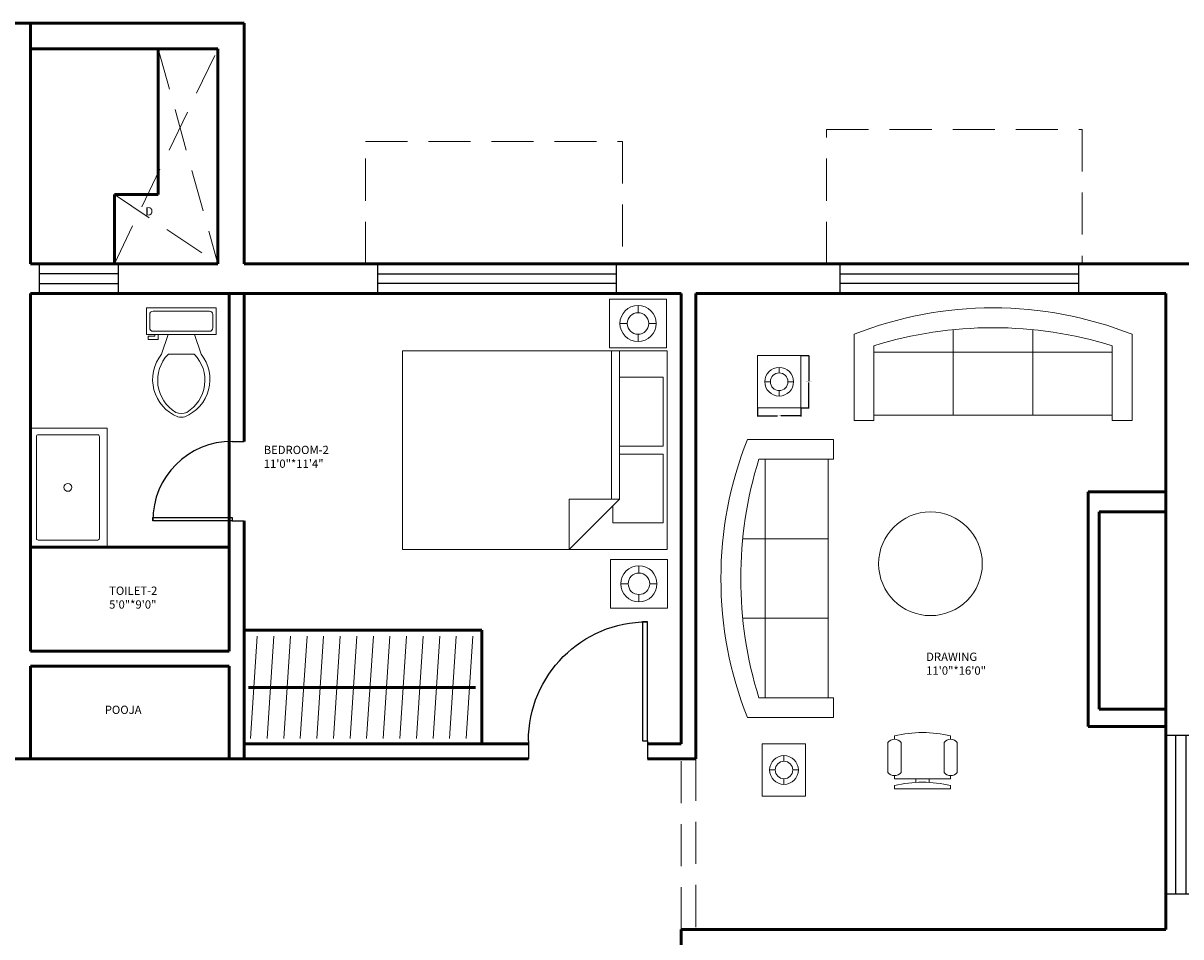
# Model space of a CAD drawing. Units: inches. Extents: x 291 to 2631, y 456 to 2623.
# Tile 3 of 22: x 550 to 900, y 728 to 1004. Entities that reach past the tile are written whole.
import ezdxf

# ---------------------------------------------------------------- set-up
doc = ezdxf.new("R2010")
doc.units = ezdxf.units.IN
doc.linetypes.add('DASHED', pattern=[19.05, 12.7, -6.35])
for name, color, linetype, lineweight in [('A-ANNO-DIMS', 2, 'Continuous', 18), ('A-ANNO-TEXT', 3, 'Continuous', 25), ('A-AREA-IDEN', 7, 'Continuous', 25), ('A-DOOR', 3, 'Continuous', 25), ('A-FLOR-FIXT', 9, 'Continuous', 18), ('A-FLOR-OVHD', 1, 'DASHED', 18), ('A-FURN', 8, 'Continuous', 18), ('A-GLAZ', 4, 'Continuous', 25), ('A-WALL', 7, 'Continuous', 50)]:
    doc.layers.add(name, color=color, linetype=linetype, lineweight=lineweight)
doc.styles.get("Standard").update_dxf_attribs({"font": 'arial.ttf'})
doc.dimstyles.get("Standard").update_dxf_attribs({"dimtxt": 0.18, "dimasz": 0.18, "dimexe": 0.18, "dimexo": 0.0625, "dimgap": 0.09, "dimtad": 0, "dimtih": 1, "dimtoh": 1, "dimdec": 4, "dimzin": 0, "dimdsep": 46, "dimtxsty": 'Standard', "dimcen": 0.09, "dimadec": 0, "dimazin": 0, "dimtfac": 1, "dimtdec": 4, "dimtofl": 0, "dimtmove": 0, "dimatfit": 3, "dimfxl": 1, "dimtolj": 1, "dimtzin": 0, "dimarcsym": 0})

# ---------------------------------------------------------------- blocks, each defined once
blk = doc.blocks.new('*U2')
for p, q in [((0, 0), (0, -6)), ((40, 0), (40, -6))]:
    blk.add_line(p, q)
blk.add_lwpolyline([(0, 0), (0, 40), (1.75, 40), (1.75, 0)], close=True)
blk.add_arc((0, 0), 40, 0, 90)
blk = doc.blocks.new('Toilet - top')
for p, q in [((9.5, -6), (9.5, -2)), ((-10, -8.5), (-8, -8.5)), ((-10, -9.5), (-10, -8.5)), ((-7, -9.5), (-10, -9.5)), ((-8, -8.5), (-8, -8)), ((-7, -8), (-7, -9.5)), ((-4, -8), (-6, -14)), ((4, -8), (6, -14)), ((4, -14), (-4, -14))]:
    blk.add_line(p, q)
blk.add_lwpolyline([(10.5, -8), (10.5, 0), (-10.5, 0), (-10.5, -8)], close=True)
for points in [[(-9.5, -2), (-9.5, -6)], [(8.5, -1), (-8.5, -1)], [(-8.5, -7), (8.5, -7)]]:
    blk.add_lwpolyline(points)
for centre, radius, start, end in [((-8.62, -1.88), 0.884, 81.8699, 188.1301), ((8.62, -1.88), 0.884, 351.8699, 98.1301), ((-8.62, -6.12), 0.884, 171.8699, 278.1301), ((8.62, -6.12), 0.884, 261.8699, 8.1301), ((3.52, -21.58), 12.17, 141.4691, 247.9714), ((4.2, -21.82), 11.33, 136.3677, 238.9468), ((-3.52, -21.58), 12.17, 292.0284, 38.5307), ((-4.2, -21.82), 11.33, 301.053, 43.6321), ((0, -27.88), 4, 245.7318, 294.2682), ((0, -29), 4, 254.8605, 285.1395)]:
    blk.add_arc(centre, radius, start, end)
blk = doc.blocks.new('Bed - Queen')
for p, q in [((0, -80.00003), (0, 0)), ((0, 0), (59.99999, 0)), ((59.99999, 0), (59.99999, -80.00003)), ((7.99999, -1.2), (28.79998, -1.2)), ((7.99999, -14.4), (7.99999, -1.2)), ((28.79998, -1.2), (28.79998, -14.4)), ((31.19999, -1.2), (51.99999, -1.2)), ((31.19999, -14.4), (31.19999, -1.2)), ((51.99999, -1.2), (51.99999, -16.4)), ((0, -14.4), (44.8, -14.4)), ((44.8, -16.8), (0, -16.8)), ((59.99999, -29.6), (44.8, -14.4)), ((44.8, -14.4), (44.8, -29.6)), ((51.99999, -16.4), (46.79936, -16.4)), ((44.8, -29.6), (59.99999, -29.6)), ((59.99999, -80.00003), (0, -80.00003))]:
    blk.add_line(p, q)
blk = doc.blocks.new('Sofa - Roundback 7 ft.')
for p, q in [((-12.00002, -32.4421), (-12.00003, -6.5971)), ((11.99997, -32.4421), (11.99998, -6.5971)), ((-36.000027, -34), (-36.000027, -11.4696)), ((-35.999844, -13.3819), (35.9998, -13.3819)), ((35.99998, -34), (35.99998, -11.4696)), ((-36.000027, -32.4421), (35.99998, -32.4421))]:
    blk.add_line(p, q)
for points in [[(-36.000027, -34), (-42.000027, -34), (-42.000027, -8)], [(41.99998, -8), (41.99998, -34), (35.99998, -34)]]:
    blk.add_lwpolyline(points)
for centre, radius, start, end in [((0, -114.25), 114.25, 68.43141, 111.5686), ((-0.00001, -127.1968), 121.1968, 72.72033, 107.2797)]:
    blk.add_arc(centre, radius, start, end)
blk = doc.blocks.new('Chair - Desk')
for p, q in [((-8.5, 0), (-8.5, -1)), ((-8.5, 0), (8.5, 0)), ((8.5, 0), (8.5, -1)), ((-8.5, -3), (-8.5, -4)), ((-8.5, -3), (8.5, -3)), ((-2, -3), (-2, -1.9355)), ((2, -1.9576), (2, -3)), ((8.5, -3), (8.5, -4)), ((-10.5, -5), (-10.5, -14)), ((-6.5, -14), (-6.5, -5)), ((6.5, -5), (6.5, -14)), ((10.5, -14), (10.5, -5)), ((-8.5, -15), (-8.5, -16)), ((8.5, -15), (8.5, -16))]:
    blk.add_line(p, q)
for centre, radius, start, end in [((0, 34.625), 36.625, 256.5803, 283.4197), ((-8.5, -6.5), 2.5, 36.8699, 143.1301), ((8.5, -6.5), 2.5, 36.8699, 143.1301), ((-8.5, -12.5), 2.5, 216.8699, 323.1301), ((0, 19.625), 36.625, 256.5803, 283.4197), ((8.5, -12.5), 2.5, 216.8699, 323.1301)]:
    blk.add_arc(centre, radius, start, end)
blk = doc.blocks.new('WIN-1800')
for p, q in [((0, 9), (72, 9)), ((0, 0), (0, 9)), ((72, 9), (72, 0)), ((0, 6), (72, 6)), ((72, 3), (0, 3)), ((72, 0), (0, 0))]:
    blk.add_line(p, q)
blk = doc.blocks.new('WIN-1200')
for p, q in [((0, 0), (0, 48)), ((0, 48), (9, 48)), ((3, 0), (3, 48)), ((6, 48), (6, 0)), ((9, 48), (9, 0)), ((9, 0), (0, 0))]:
    blk.add_line(p, q)
blk = doc.blocks.new('WIN-600')
for p, q in [((24, 9), (0, 9)), ((0, 9), (0, 0)), ((24, 0), (24, 9)), ((24, 6), (0, 6)), ((0, 3), (24, 3)), ((0, 0), (24, 0))]:
    blk.add_line(p, q)
blk = doc.blocks.new('LAMP-A')
for p, q in [((6.55, 12.25), (6.55, 10.56)), ((2.2, 7.9), (3.88, 7.9)), ((9.21, 7.9), (10.89, 7.9)), ((6.55, 5.24), (6.55, 3.56))]:
    blk.add_line(p, q)
blk.add_lwpolyline([(0, 15.8), (13.09, 15.8), (13.09, 0), (0, 0)], close=True)
for radius in [4.34, 2.66]:
    blk.add_circle((6.55, 7.9), radius)
blk = doc.blocks.new('LAMP-B')
for p, q in [((8.62, 12.82), (8.62, 10.61)), ((3.15, 7.36), (5.36, 7.36)), ((11.87, 7.36), (14.08, 7.36)), ((8.62, 4.1), (8.62, 1.89))]:
    blk.add_line(p, q)
blk.add_lwpolyline([(0, 14.71), (17.23, 14.71), (17.23, 0), (0, 0)], close=True)
for radius in [5.46, 3.25]:
    blk.add_circle((8.62, 7.36), radius)
blk = doc.blocks.new('*D38')
at = {"layer": 'A-ANNO-DIMS', "color": 0, "lineweight": -2, "transparency": 16777216}
for p, q in [((784.77, 903.25), (787.25, 903.25)), ((787.07, 903.07), (787.07, 895.53)), ((787.07, 887.63), (787.07, 895.17)), ((784.77, 887.45), (787.25, 887.45))]:
    blk.add_line(p, q, dxfattribs=at)
at = {"layer": 'A-ANNO-DIMS', "color": 0, "transparency": 16777216}
for points in [[(787.04, 903.07), (787.1, 903.07), (787.07, 903.25)], [(787.04, 887.63), (787.1, 887.63), (787.07, 887.45)]]:
    blk.add_solid(points, dxfattribs=at)
at = {"layer": 'DEFPOINTS', "color": 0, "transparency": 16777216}
for p in [(784.7, 903.25), (787.07, 903.25), (784.7, 887.45)]:
    blk.add_point(p, dxfattribs=at)
at = {"layer": 'A-ANNO-DIMS', "color": 0, "transparency": 16777216, "insert": (787.07, 895.35), "char_height": 0.18, "attachment_point": 5}
blk.add_mtext('\\A1;LAMP A 16 TYP.', dxfattribs=at)
blk = doc.blocks.new('*D39')
at = {"layer": 'A-ANNO-DIMS', "color": 0, "lineweight": -2, "transparency": 16777216}
for p, q in [((771.61, 887.39), (771.61, 884.9)), ((771.79, 885.08), (777.64, 885.08)), ((784.52, 885.08), (778.68, 885.08)), ((784.7, 887.39), (784.7, 884.9))]:
    blk.add_line(p, q, dxfattribs=at)
at = {"layer": 'A-ANNO-DIMS', "color": 0, "transparency": 16777216}
for points in [[(771.79, 885.11), (771.79, 885.05), (771.61, 885.08)], [(784.52, 885.11), (784.52, 885.05), (784.7, 885.08)]]:
    blk.add_solid(points, dxfattribs=at)
at = {"layer": 'DEFPOINTS', "color": 0, "transparency": 16777216}
for p in [(771.61, 887.45), (784.7, 887.45), (784.7, 885.08)]:
    blk.add_point(p, dxfattribs=at)
at = {"layer": 'A-ANNO-DIMS', "color": 0, "transparency": 16777216, "insert": (778.16, 885.08), "char_height": 0.18, "attachment_point": 5}
blk.add_mtext('\\A1;13 TYP.', dxfattribs=at)

msp = doc.modelspace()

# ---------------------------------------------------------------- linework, layer by layer
at = {"layer": 'A-FLOR-OVHD'}
for p, q in [((577.32, 930.98), (608.57, 995.89)), ((590.53, 995.89), (608.57, 930.98)), ((792.48, 930.98), (792.48, 971.52)), ((792.48, 971.52), (869.7, 971.52)), ((869.7, 971.52), (869.7, 930.98)), ((653.15, 930.98), (653.15, 967.92)), ((653.15, 967.92), (730.86, 967.92)), ((730.86, 967.92), (730.86, 930.98)), ((577.32, 951.91), (608.57, 930.98)), ((748.5, 729.98), (748.5, 781.48)), ((753, 781.48), (753, 729.98))]:
    msp.add_line(p, q, dxfattribs=at)
at = {"layer": 'A-FURN'}
for p, q in [((618.45, 787.61), (620.48, 818.48)), ((623.46, 787.61), (625.49, 818.48)), ((628.47, 787.61), (630.5, 818.48)), ((633.48, 787.61), (635.51, 818.48)), ((638.5, 787.61), (640.52, 818.48)), ((643.51, 787.61), (645.53, 818.48)), ((648.52, 787.61), (650.54, 818.48)), ((653.53, 787.61), (655.56, 818.48)), ((658.54, 787.61), (660.57, 818.48)), ((663.55, 787.61), (665.58, 818.48)), ((668.56, 787.61), (670.59, 818.48)), ((673.58, 787.61), (675.6, 818.48)), ((678.59, 787.61), (680.61, 818.48)), ((683.6, 787.61), (685.62, 818.48))]:
    msp.add_line(p, q, dxfattribs=at)
msp.add_lwpolyline([(552, 845.35), (575.09, 845.35), (575.09, 881.35), (552, 881.35)], close=True, dxfattribs=at)
msp.add_lwpolyline([(554.24, 879.34), (572.3, 879.34, -0.414214), (572.8, 878.84), (572.8, 848.05, -0.414214), (572.3, 847.55), (554.24, 847.55, -0.414214), (553.74, 848.05), (553.74, 878.84, -0.414214)], format="xyb", close=True, dxfattribs=at)
for centre, radius in [((563.27, 863.44), 1.18), ((823.86, 840.39), 15.66)]:
    msp.add_circle(centre, radius, dxfattribs=at)
at = {"layer": 'A-WALL'}
for p, q in [((483.37, 1003.63), (616.5, 1003.63)), ((552, 930.98), (552, 1003.63)), ((616.5, 1003.63), (616.5, 930.98)), ((552, 995.89), (608.57, 995.89)), ((590.53, 951.91), (590.53, 995.89)), ((608.57, 995.89), (608.57, 930.98)), ((577.32, 930.98), (577.32, 951.91)), ((577.32, 951.91), (590.53, 951.91)), ((608.57, 930.98), (552, 930.98)), ((904, 930.98), (616.5, 930.98)), ((552, 862.1), (552, 921.98)), ((748.5, 921.98), (552, 921.98)), ((612, 813.98), (612, 921.98)), ((616.5, 877.35), (616.5, 921.98)), ((748.5, 862.1), (748.5, 921.98)), ((895, 921.98), (753, 921.98)), ((753, 862.1), (753, 921.98)), ((895, 862.1), (895, 921.98)), ((552, 862.1), (552, 813.98)), ((748.5, 862.1), (748.5, 785.98)), ((753, 862.1), (753, 781.48)), ((895, 862.1), (871.5, 862.1)), ((871.5, 862.1), (871.5, 791.23)), ((895, 862.1), (895, 729.98)), ((895, 856.09), (874.84, 856.09)), ((874.84, 856.09), (874.84, 796.46)), ((616.5, 781.48), (616.5, 853.35)), ((552, 845.35), (612, 845.35)), ((616.5, 820.36), (688.34, 820.36)), ((688.34, 820.36), (688.34, 785.98)), ((612, 813.98), (552, 813.98)), ((612, 809.48), (552, 809.48)), ((552, 809.48), (552, 781.48)), ((612, 781.48), (612, 809.48)), ((617.86, 803.04), (686.43, 803.04)), ((874.84, 796.46), (895, 796.46)), ((871.5, 791.23), (895, 791.23)), ((702.4, 785.98), (616.5, 785.98)), ((748.5, 785.98), (738.4, 785.98)), ((702.4, 781.48), (539.53, 781.48)), ((753, 781.48), (738.4, 781.48)), ((895, 729.98), (748.5, 729.98)), ((748.5, 729.98), (748.5, 682.38))]:
    msp.add_line(p, q, dxfattribs=at)

# ---------------------------------------------------------------- block references
at = {"layer": 'A-DOOR', "xscale": 0.6, "yscale": 0.6, "zscale": 0.6, "rotation": 90.00000000000003}
msp.add_blockref('*U2', (612.9, 853.35), dxfattribs=at)
at = {"layer": 'A-DOOR', "xscale": -0.9, "yscale": 0.9, "zscale": 0.9}
msp.add_blockref('*U2', (738.4, 786.88), dxfattribs=at)
at = {"layer": 'A-FLOR-FIXT'}
msp.add_blockref('Toilet - top', (597.52, 917.63), dxfattribs=at)
at = {"layer": 'A-FURN'}
for name, p in [('LAMP-B', (726.89, 905.58)), ('Sofa - Roundback 7 ft.', (842.76, 917.67)), ('LAMP-A', (771.61, 887.45)), ('LAMP-B', (727.16, 826.98)), ('LAMP-A', (773.06, 770.21))]:
    msp.add_blockref(name, p, dxfattribs=at)
for name, p, rotation in [('Bed - Queen', (744.31, 904.7), 270), ('Sofa - Roundback 7 ft.', (760.55, 835.93), 89.99999999999999), ('Chair - Desk', (821.46, 772.4), 180)]:
    msp.add_blockref(name, p, dxfattribs=dict(at, rotation=rotation))
at = {"layer": 'A-GLAZ', "rotation": 180}
msp.add_blockref('WIN-600', (578.57, 930.98), dxfattribs=at)
at = {"layer": 'A-GLAZ'}
for name, p in [('WIN-1800', (656.91, 921.98)), ('WIN-1800', (796.55, 921.98)), ('WIN-1200', (895, 740.63))]:
    msp.add_blockref(name, p, dxfattribs=at)

# ---------------------------------------------------------------- texts
at = {"layer": 'A-ANNO-TEXT', "insert": (586.67, 948.07), "char_height": 2.5, "attachment_point": 1}
msp.add_mtext_dynamic_manual_height_columns('D', width=5.0576, gutter_width=12.5, heights=[0], dxfattribs=at)
at = {"layer": 'A-AREA-IDEN', "char_height": 2.5, "attachment_point": 1}
for s, width, insert in [('BEDROOM-2\\P11\'0"*11\'4"', 37.7818, (622.43, 876.02)), ('TOILET-2\\P5\'0"*9\'0"', 42.4349, (575.73, 833.5)), ('DRAWING\\P11\'0"*16\'0"', 48.3574, (822.56, 813.55)), ('POOJA', 42.118, (574.41, 797.53))]:
    msp.add_mtext_dynamic_manual_height_columns(s, width=width, gutter_width=12.5, heights=[0], dxfattribs=dict(at, insert=insert))

# ---------------------------------------------------------------- dimensions: what is measured, and where the dimension line sits
at = {"layer": 'A-ANNO-DIMS'}
dim = msp.add_linear_dim(base=(787.07, 903.25), p1=(784.7, 887.45), p2=(784.7, 903.25), angle=90, text='LAMP A <> TYP.', dimstyle='Standard', override={"dimdec": 0, "dimlfac": 1, "dimrnd": 0, "dimzin": 0, "dimdsep": 46, "dimlunit": 2}, dxfattribs=at)
dim.commit()
dim.dimension.update_dxf_attribs({"geometry": '*D38', "text_midpoint": (787.07, 895.35)})
dim = msp.add_linear_dim(base=(784.7, 885.08), p1=(771.61, 887.45), p2=(784.7, 887.45), text='<> TYP.', dimstyle='Standard', override={"dimdec": 0, "dimlfac": 1, "dimrnd": 0, "dimzin": 0, "dimdsep": 46, "dimlunit": 2}, dxfattribs=at)
dim.commit()
dim.dimension.update_dxf_attribs({"geometry": '*D39', "text_midpoint": (778.16, 885.08)})

doc.saveas('drawing.dxf')
